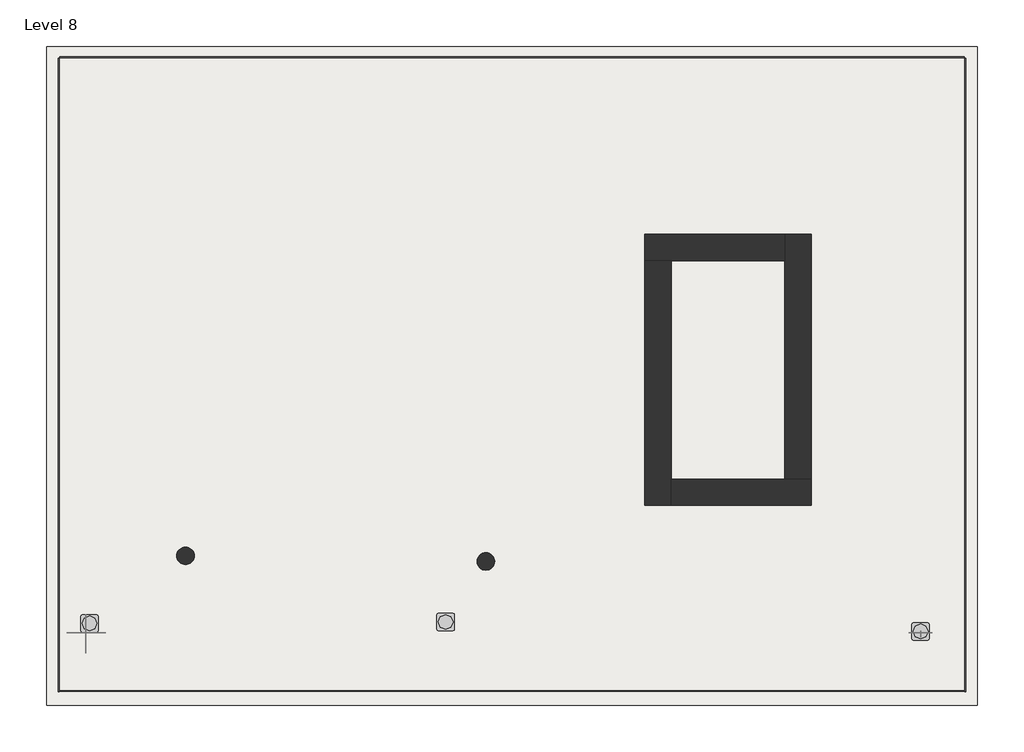
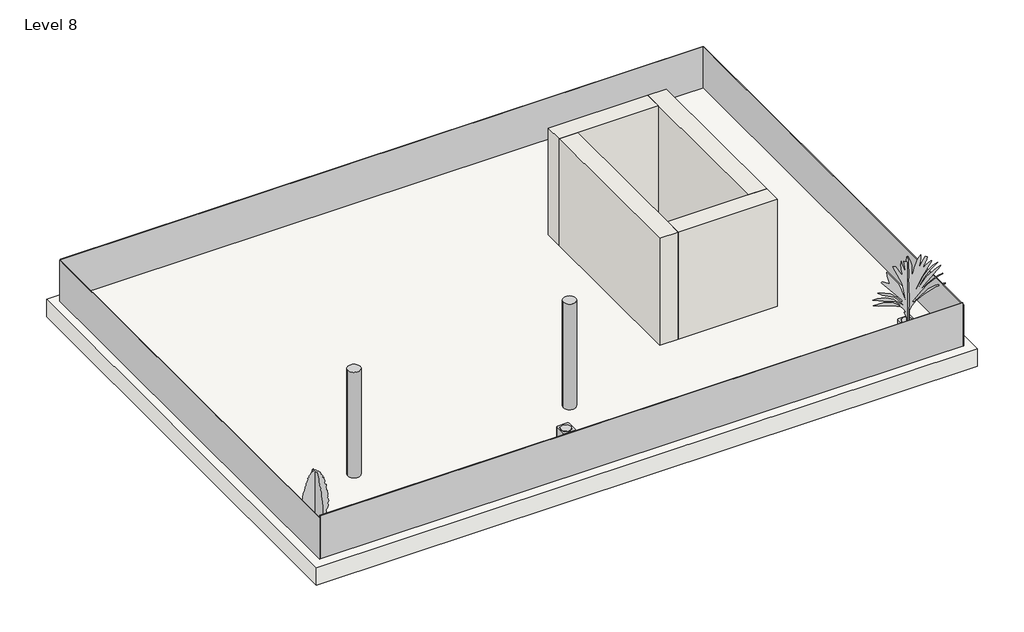
# One storey, incomplete: 4 plates, 4 walls, 3 proxies, 2 columns, 2 geographic elements, 1 slab.
"""IFC4 building model written with IfcOpenShell, lengths in millimetres."""

from ifc_helpers import new_model, si_unit, frame, origin, place, context, project, spatial, polyline, outline, extrude, faceted_brep, transform, mapped, element, save
from components import proxy_13b82c07, column_dfe452ed, rpc_tree_conifer_chinese_juniper_7_5155a079, rpc_tree_tropical_0177ab4a, system_panel_glazed_ba49168f, system_panel_glazed_f2f268b4, system_panel_glazed_f8a0c966, system_panel_glazed_fd840cde

model = new_model("IFC4")

# Units and contexts
model_context = context("Model", 3, world=origin())
ifc_project = project(units=[si_unit("LENGTHUNIT", "METRE", prefix="MILLI")], contexts=[model_context])

# Site, building, storey
site = spatial("IfcSite", under=ifc_project)
building = spatial("IfcBuilding", under=site)
storey = spatial("IfcBuildingStorey", under=building, Name="Level 8", Elevation=21336.0)

# Proxies
placement = place(None, origin())
proxy_shape = proxy_13b82c07(model_context)
element("IfcBuildingElementProxy", 1, Name="Air Conditioner-Outside Unit : 33\" x 24\" x 24\"", ObjectType="Air Conditioner-Outside Unit : 33\" x 24\" x 24\"", at=placement, inside=storey, context=model_context, shape_type="MappedRepresentation", body=[
    mapped(proxy_shape, transform((-24603.5874719, -2613.1632813, 21031.2), x_axis=(1.0, 0.0, 0.0), y_axis=(0.0, 1.0, 0.0), z_axis=(0.0, 0.0, 1.0))),
])
element("IfcBuildingElementProxy", 2, Name="Air Conditioner-Outside Unit : 33\" x 24\" x 24\"", ObjectType="Air Conditioner-Outside Unit : 33\" x 24\" x 24\"", at=placement, inside=storey, context=model_context, shape_type="MappedRepresentation", body=[
    mapped(proxy_shape, transform((4377.8125281, -2892.5632813, 21031.2), x_axis=(1.0, 0.0, 0.0), y_axis=(0.0, 1.0, 0.0), z_axis=(0.0, 0.0, 1.0))),
])
element("IfcBuildingElementProxy", 3, Name="Air Conditioner-Outside Unit : 33\" x 24\" x 24\"", ObjectType="Air Conditioner-Outside Unit : 33\" x 24\" x 24\"", at=placement, inside=storey, context=model_context, shape_type="MappedRepresentation", body=[
    mapped(proxy_shape, transform((-12182.9874719, -2562.3632813, 21031.2), x_axis=(1.0, 0.0, 0.0), y_axis=(0.0, 1.0, 0.0), z_axis=(0.0, 0.0, 1.0))),
])

# Columns
column_shape = column_dfe452ed(model_context)
element("IfcColumn", 4, ObjectType="Round Column : 24\" Diameter", at=placement, inside=storey, context=model_context, shape_type="MappedRepresentation", body=[
    mapped(column_shape, transform((-24398.13551, -4657.6708522, 0.0), x_axis=(1.0, 0.0, 0.0), y_axis=(0.0, 1.0, 0.0), z_axis=(0.0, 0.0, 1.0))),
])
element("IfcColumn", 5, ObjectType="Round Column : 24\" Diameter", at=placement, inside=storey, context=model_context, shape_type="MappedRepresentation", body=[
    mapped(column_shape, transform((-13927.1724365, -4854.7077787, 0.0), x_axis=(1.0, 0.0, 0.0), y_axis=(0.0, 1.0, 0.0), z_axis=(0.0, 0.0, 1.0))),
])

# Geographic elements
rpc_tree_conifer_chinese_juniper_7_shape = rpc_tree_conifer_chinese_juniper_7_5155a079(model_context)
element("IfcGeographicElement", 6, ObjectType="RPC Tree - Conifer : Chinese Juniper - 7'", at=placement, inside=storey, context=model_context, shape_type="MappedRepresentation", body=[
    mapped(rpc_tree_conifer_chinese_juniper_7_shape, transform((-24730.784143, -2943.3632813, 21031.2), x_axis=(1.0, 0.0, 0.0), y_axis=(0.0, 1.0, 0.0), z_axis=(0.0, 0.0, 1.0))),
])
rpc_tree_tropical_shape = rpc_tree_tropical_0177ab4a(model_context)
element("IfcGeographicElement", 7, ObjectType="RPC Tree - Tropical", at=placement, inside=storey, context=model_context, shape_type="MappedRepresentation", body=[
    mapped(rpc_tree_tropical_shape, transform((4377.8125281, -2943.3632813, 21031.2), x_axis=(1.0, 0.0, 0.0), y_axis=(0.0, 1.0, 0.0), z_axis=(0.0, 0.0, 1.0))),
])

# Plates
system_panel_glazed_shape = system_panel_glazed_ba49168f(model_context)
element("IfcPlate", 8, ObjectType="System Panel : Glazed", at=placement, inside=storey, context=model_context, shape_type="MappedRepresentation", body=[
    mapped(system_panel_glazed_shape, transform((-25644.9874719, 6048.2367187, 21031.2), x_axis=(0.0, 1.0, 0.0), y_axis=(-1.0, 0.0, 0.0), z_axis=(0.0, 0.0, 1.0))),
])
system_panel_glazed_2_shape = system_panel_glazed_f2f268b4(model_context)
element("IfcPlate", 9, ObjectType="System Panel : Glazed", at=placement, inside=storey, context=model_context, shape_type="MappedRepresentation", body=[
    mapped(system_panel_glazed_2_shape, transform((-9871.5874719, 17097.2367187, 21031.2), x_axis=(1.0, 0.0, 0.0), y_axis=(0.0, 1.0, 0.0), z_axis=(0.0, 0.0, 1.0))),
])
system_panel_glazed_3_shape = system_panel_glazed_f8a0c966(model_context)
element("IfcPlate", 10, ObjectType="System Panel : Glazed", at=placement, inside=storey, context=model_context, shape_type="MappedRepresentation", body=[
    mapped(system_panel_glazed_3_shape, transform((5901.8125281, 6048.2367187, 21031.2), x_axis=(0.0, -1.0, 0.0), y_axis=(1.0, 0.0, 0.0), z_axis=(0.0, 0.0, 1.0))),
])
system_panel_glazed_4_shape = system_panel_glazed_fd840cde(model_context)
element("IfcPlate", 11, ObjectType="System Panel : Glazed", at=placement, inside=storey, context=model_context, shape_type="MappedRepresentation", body=[
    mapped(system_panel_glazed_4_shape, transform((-9871.5874719, -5000.7632813, 21031.2), x_axis=(1.0, 0.0, 0.0), y_axis=(0.0, 1.0, 0.0), z_axis=(0.0, 0.0, 1.0))),
])

# Slab
element("IfcSlab", 12, ObjectType="Generic - 3'", at=placement, inside=storey, context=model_context, shape_type="SweptSolid", body=[
    extrude(outline(polyline([(-26102.1874719, -5457.9632813), (-26102.1874719, 17503.6367187), (6359.0125281, 17503.6367187), (6359.0125281, -5457.9632813), (-26102.1874719, -5457.9632813)])), frame((0.0, 0.0, 20116.8), z_axis=(0.0, 0.0, 1.0), x_axis=(1.0, 0.0, 0.0)), (0.0, 0.0, 1.0), 914.4),
])

# Walls
element("IfcWall", 13, ObjectType="Generic - 3'", at=placement, inside=storey, context=model_context, shape_type="Brep", body=[
    faceted_brep([(557.1720609, 2421.4679902, 21031.2), (-4319.6279391, 2421.4679902, 21031.2), (-4319.6279391, 2421.4679902, 26584.2329136), (-357.2279391, 2421.4679902, 26584.2329136), (557.1720609, 2421.4679902, 26584.2329136), (557.1720609, 1507.0679902, 21031.2), (557.1720609, 1507.0679902, 26584.2329136), (-4319.6279391, 1507.0679902, 26584.2329136), (-4319.6279391, 1507.0679902, 21031.2)], [[[0, 1, 2, 3, 4]], [[5, 6, 7, 8]], [[1, 0, 5, 8]], [[4, 3, 2, 7, 6]], [[0, 4, 6, 5]], [[2, 1, 8, 7]]]),
])
element("IfcWall", 14, ObjectType="Generic - 3'", at=placement, inside=storey, context=model_context, shape_type="Brep", body=[
    faceted_brep([(-357.2279391, 10955.8679902, 20690.1677574), (-357.2279391, 2421.4679902, 20690.1677574), (-357.2279391, 2421.4679902, 26584.2329136), (-357.2279391, 10041.4679902, 26584.2329136), (-357.2279391, 10955.8679902, 26584.2329136), (557.1720609, 10955.8679902, 20690.1677574), (557.1720609, 10955.8679902, 26584.2329136), (557.1720609, 2421.4679902, 26584.2329136), (557.1720609, 2421.4679902, 21031.2), (557.1720609, 2421.4679902, 20690.1677574)], [[[0, 1, 2, 3, 4]], [[5, 6, 7, 8, 9]], [[1, 0, 5, 9]], [[4, 3, 2, 7, 6]], [[0, 4, 6, 5]], [[2, 1, 9, 8, 7]]]),
])
element("IfcWall", 15, ObjectType="Generic - 3'", at=placement, inside=storey, context=model_context, shape_type="Brep", body=[
    faceted_brep([(-5234.0279391, 10041.4679902, 20084.6383385), (-357.2279391, 10041.4679902, 20084.6383385), (-357.2279391, 10041.4679902, 26584.2329136), (-5234.0279391, 10041.4679902, 26584.2329136), (-5234.0279391, 10041.4679902, 21031.2), (-5234.0279391, 10955.8679902, 20084.6383385), (-5234.0279391, 10955.8679902, 26584.2329136), (-357.2279391, 10955.8679902, 26584.2329136), (-357.2279391, 10955.8679902, 20690.1677574), (-357.2279391, 10955.8679902, 20084.6383385)], [[[0, 1, 2, 3, 4]], [[5, 6, 7, 8, 9]], [[1, 0, 5, 9]], [[3, 2, 7, 6]], [[0, 4, 3, 6, 5]], [[2, 1, 9, 8, 7]]]),
])
element("IfcWall", 16, ObjectType="Generic - 3'", at=placement, inside=storey, context=model_context, shape_type="Brep", body=[
    faceted_brep([(-4319.6279391, 1507.0679902, 21031.2), (-4319.6279391, 2421.4679902, 21031.2), (-4319.6279391, 10041.4679902, 21031.2), (-4319.6279391, 10041.4679902, 26587.7994419), (-4319.6279391, 1507.0679902, 26587.7994419), (-4319.6279391, 1507.0679902, 26584.2329136), (-5234.0279391, 1507.0679902, 21031.2), (-5234.0279391, 1507.0679902, 26587.7994419), (-5234.0279391, 10041.4679902, 26587.7994419), (-5234.0279391, 10041.4679902, 26584.2329136), (-5234.0279391, 10041.4679902, 21031.2)], [[[0, 1, 2, 3, 4, 5]], [[6, 7, 8, 9, 10]], [[2, 1, 0, 6, 10]], [[4, 3, 8, 7]], [[0, 5, 4, 7, 6]], [[3, 2, 10, 9, 8]]]),
])

save(model, "model.ifc")

# Revit data of these elements
# Type "Air Conditioner-Outside Unit : 33\" x 24\" x 24\""
#   Assembly Code = "D3030"
#   Depth = 2' - 0"
#   Height = 2' - 0"
#   Width = 2' - 0"
#   Air Conditioner Material = Steel, Paint Finish, Dark Gray, Matte
#   Default Elevation = 0
# Type "Round Column : 24\" Diameter"
#   Assembly Code = "B1010200"
#   Diameter = 2' - 0"
#   Offset Base = 0' - 0"
#   Offset Top = 0' - 0"
#   Material = none
# Type "RPC Tree - Conifer : Chinese Juniper - 7'"
#   built-in parameter 1005198 = "{2, 15},{39, RPC-16-FUM3-UUQ0-UBF0-N000-ST1L-LVER-AU},{1, 0},{1, 0},{2, 13},{1, 8},{5, Color},{1, 0},{1, 0},{3, 0.8},{3, 0.8},{3, 0.8},{1, 8},{7, BBoxMin},{1, 0},{1, 0},{1, 0},{1, 0},{1, 0},{1, 8},{7, BBoxMax},{1, 0},{1, 0},{1, 0},{1, 0},{1, 0},{2, 11},{9, RPCTypeId},{1, 0},{1, 0},{39, RPC-16-FUM3-UUQ0-UBF0-N000-ST1L-LVER-AU},{1, 6},{14, RPCPlantHeight},{1, 0},{1, 0},{1, 7},{2, 11},{7, keyword},{1, 0},{1, 0},{34, :RPCs:Trees [General]:Geometry:RPC},{2, 11},{8, category},{1, 0},{1, 0},{15, Trees [General]},{2, 11},{12, LocalizedUID},{1, 0},{1, 0},{15, Chinese Juniper},{2, 14},{6, Height},{1, 0},{1, 0},{1, 7},{1, 2},{16, Cast Reflections},{1, 0},{1, 0},{1, 0},{1, 2},{12, Cast Shadows},{1, 0},{1, 0},{1, 1},{1, 2},{9, Lock View},{1, 0},{1, 0},{1, 0},{1, 4},{5, ViewC},{1, 0},{1, 0},{1, 0},{21, assetlibrary_base.fbx},{1, 5},"
#   built-in parameter 1005195 = "RPC-16-FUM3-UUQ0-UBF0-N000-ST1L-LVER-AU"
#   Type Comments = "Chinese Juniper"
#   Assembly Code = "G2050500"
#   Height = 10' - 0"
#   Description = (empty or 0)
#   Default Elevation = 0
# Type "RPC Tree - Tropical"
#   built-in parameter 1005198 = "{2, 15},{39, RPC-16-G2M6-EAFX-C5H6-W000-ST1L-LVER-AU},{1, 0},{1, 0},{2, 13},{1, 8},{5, Color},{1, 0},{1, 0},{3, 0.8},{3, 0.8},{3, 0.8},{1, 8},{7, BBoxMin},{1, 0},{1, 0},{1, 0},{1, 0},{1, 0},{1, 8},{7, BBoxMax},{1, 0},{1, 0},{1, 0},{1, 0},{1, 0},{2, 11},{9, RPCTypeId},{1, 0},{1, 0},{39, RPC-16-G2M6-EAFX-C5H6-W000-ST1L-LVER-AU},{1, 6},{14, RPCPlantHeight},{1, 0},{1, 0},{2, 13},{2, 11},{7, keyword},{1, 0},{1, 0},{35, :RPCs:Trees [Tropical]:Geometry:RPC},{2, 11},{8, category},{1, 0},{1, 0},{16, Trees [Tropical]},{2, 11},{12, LocalizedUID},{1, 0},{1, 0},{15, Traveler's Palm},{2, 14},{6, Height},{1, 0},{1, 0},{2, 13},{1, 2},{16, Cast Reflections},{1, 0},{1, 0},{1, 0},{1, 2},{12, Cast Shadows},{1, 0},{1, 0},{1, 1},{1, 2},{9, Lock View},{1, 0},{1, 0},{1, 0},{1, 4},{5, ViewC},{1, 0},{1, 0},{1, 0},{21, assetlibrary_base.fbx},{1, 5},"
#   built-in parameter 1005195 = "RPC-16-G2M6-EAFX-C5H6-W000-ST1L-LVER-AU"
#   Assembly Code = "G2050500"
#   Height = 13' - 0"
#   Plan Symbol = element 321958
#   Default Elevation = 0
# Type "System Panel : Glazed"
#   Construction Type Id = "GSP4R"
#   Analytic Construction = "1/8 in Pilkington single glazing"
#   Visual Light Transmittance = 0.9
#   Solar Heat Gain Coefficient = 0.86
#   Heat Transfer Coefficient (U) = 1.18115 BTU/(h·ft²·°F)
# Type "Generic - 3'"
#   Assembly Code = "B1010"
#   Function = 0
#   Layers, outside or top first: 3' - 0" "Parking Stripe" (function 1)
# Type "Generic - 3'"
#   Assembly Code = "B2010"
#   Layers, outside or top first: 3' - 0" "Parking Stripe" (function 1)
# Element 1 (IfcBuildingElementProxy, "Air Conditioner-Outside Unit : 33\" x 24\" x 24\"")
#   Mark = "10"
#   Phase Created = New Construction
#   Materials on its faces: "Steel, Paint Finish, Dark Gray, Matte"
# Element 2 (IfcBuildingElementProxy, "Air Conditioner-Outside Unit : 33\" x 24\" x 24\"")
#   Mark = "11"
#   Phase Created = New Construction
#   Materials on its faces: "Steel, Paint Finish, Dark Gray, Matte"
# Element 3 (IfcBuildingElementProxy, "Air Conditioner-Outside Unit : 33\" x 24\" x 24\"")
#   Mark = "12"
#   Phase Created = New Construction
#   Materials on its faces: "Steel, Paint Finish, Dark Gray, Matte"
# Elements 4, 5 (IfcColumn, "Round Column : 24\" Diameter")
#   Phase Created = New Construction
# Element 6 (IfcGeographicElement, "RPC Tree - Conifer : Chinese Juniper - 7'")
#   Phase Created = New Construction
# Element 7 (IfcGeographicElement, "RPC Tree - Tropical")
#   Phase Created = New Construction
# Elements 8, 9, 10, 11 (IfcPlate, "System Panel : Glazed")
#   Phase Created = New Construction
#   Materials on its faces: "Glass"
# Element 12 (IfcSlab, "Generic - 3'")
#   built-in parameter 1001955 = 3.14159 (stored number, unit not read)
#   Height Offset From Level = -1' - 0"
#   Phase Created = New Construction
#   Materials on its faces: "Parking Stripe"
# Element 13 (IfcWall, "Generic - 3'")
#   built-in parameter 1001111 = -1' - 0"
#   Top Offset = 0' - 0"
#   Base Offset = -1' - 0"
#   Unconnected Height = 18' - 2.62334"
#   wall height = 18' - 2.62334"
#   Phase Created = New Construction
#   Base Constraint = Level 8
#   Materials on its faces: "Parking Stripe"
# Element 14 (IfcWall, "Generic - 3'")
#   built-in parameter 1001111 = -2' - 1.42647"
#   Top Offset = 0' - 0"
#   Base Offset = -2' - 1.42647"
#   Unconnected Height = 19' - 4.04981"
#   wall height = 19' - 4.04981"
#   Phase Created = New Construction
#   Base Constraint = Level 8
#   Materials on its faces: "Parking Stripe"
# Element 15 (IfcWall, "Generic - 3'")
#   built-in parameter 1001111 = -4' - 1.26621"
#   Top Offset = 0' - 0"
#   Base Offset = -4' - 1.26621"
#   Unconnected Height = 21' - 3.88955"
#   wall height = 21' - 3.88955"
#   Phase Created = New Construction
#   Base Constraint = Level 8
#   Materials on its faces: "Parking Stripe"
# Element 16 (IfcWall, "Generic - 3'")
#   built-in parameter 1001111 = -1' - 0"
#   Top Offset = 0' - 0"
#   Base Offset = -1' - 0"
#   Unconnected Height = 18' - 2.76376"
#   wall height = 18' - 2.76376"
#   Phase Created = New Construction
#   Base Constraint = Level 8
#   Materials on its faces: "Parking Stripe"
# Materials
#   "Steel, Paint Finish, Dark Gray, Matte": class "Metal", colour RGB 98 98 98, transparency 0, Description = "Steel, paint finish, dark gray, matte", Cost = 0
#   "Parking Stripe": class "Paint", colour RGB 250 250 91, transparency 0, Cost = 0
#   "Glass": class "Glass", colour RGB 0 128 192, transparency 0.75, Description = "Soda Lime Glass", Cost = 0
